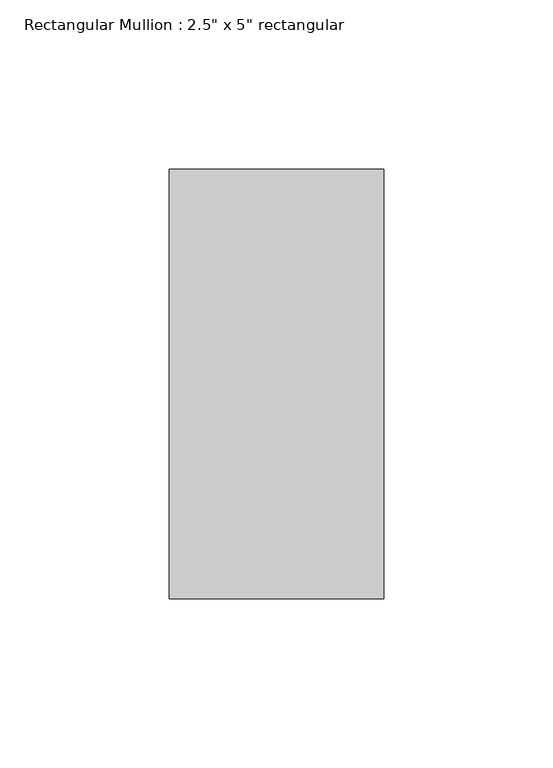
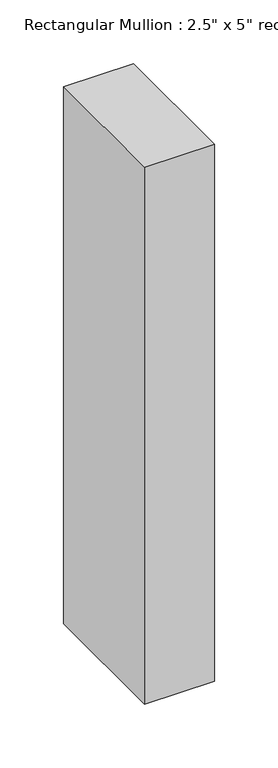
"""IFC4 building model written with IfcOpenShell, lengths in millimetres: member geometry."""

from ifc_helpers import new_model, si_unit, frame, origin, place, context, project, spatial, polyline, outline, extrude, source, transform, mapped, element, save


def member_0b7646a3(model_context):
    return source(origin(), model_context, "Body", "SweptSolid", [
        extrude(outline(polyline([(0.0, 63.5), (0.0, -63.5), (-63.5, -63.5), (-63.5, 63.5), (0.0, 63.5)])), frame((0.0, 0.0, -514.35), z_axis=(0.0, 0.0, 1.0), x_axis=(1.0, 0.0, 0.0)), (0.0, 0.0, 1.0), 514.35),
    ])


if __name__ == "__main__":
    model = new_model("IFC4")
    model_context = context("Model", 3, world=origin())
    ifc_project = project(units=[si_unit("LENGTHUNIT", "METRE", prefix="MILLI")], contexts=[model_context])
    site = spatial("IfcSite", under=ifc_project)
    building = spatial("IfcBuilding", under=site)
    placement = place(None, origin())
    member_shape = member_0b7646a3(model_context)
    element("IfcMember", 1, ObjectType="Rectangular Mullion : 2.5\" x 5\" rectangular", at=placement, inside=building, context=model_context, shape_type="MappedRepresentation", body=[
        mapped(member_shape, transform((0.0, 0.0, 0.0), x_axis=(1.0, 0.0, 0.0), y_axis=(0.0, 1.0, 0.0), z_axis=(0.0, 0.0, 1.0))),
    ])
    save(model, "model.ifc")

# Revit data of these elements
# Type "Rectangular Mullion : 2.5\" x 5\" rectangular"
#   built-in parameter 1007304 = 0.416667 (stored number, unit not read)
#   built-in parameter 1007301 = 0.104167 (stored number, unit not read)
#   built-in parameter 1007300 = 0.104167 (stored number, unit not read)
# Element 1 (IfcMember, "Rectangular Mullion : 2.5\" x 5\" rectangular")
#   Materials on its faces: "Aluminum"
# Materials
#   "Aluminum": class "Metal", colour RGB 247 247 247, transparency 0, Description = "Aluminum 6061", Cost = 0
